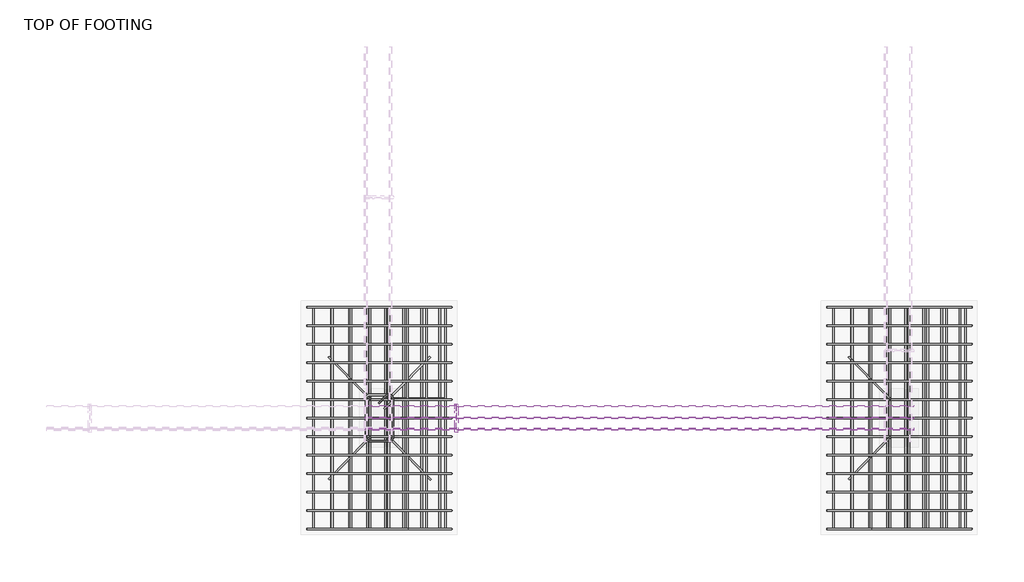
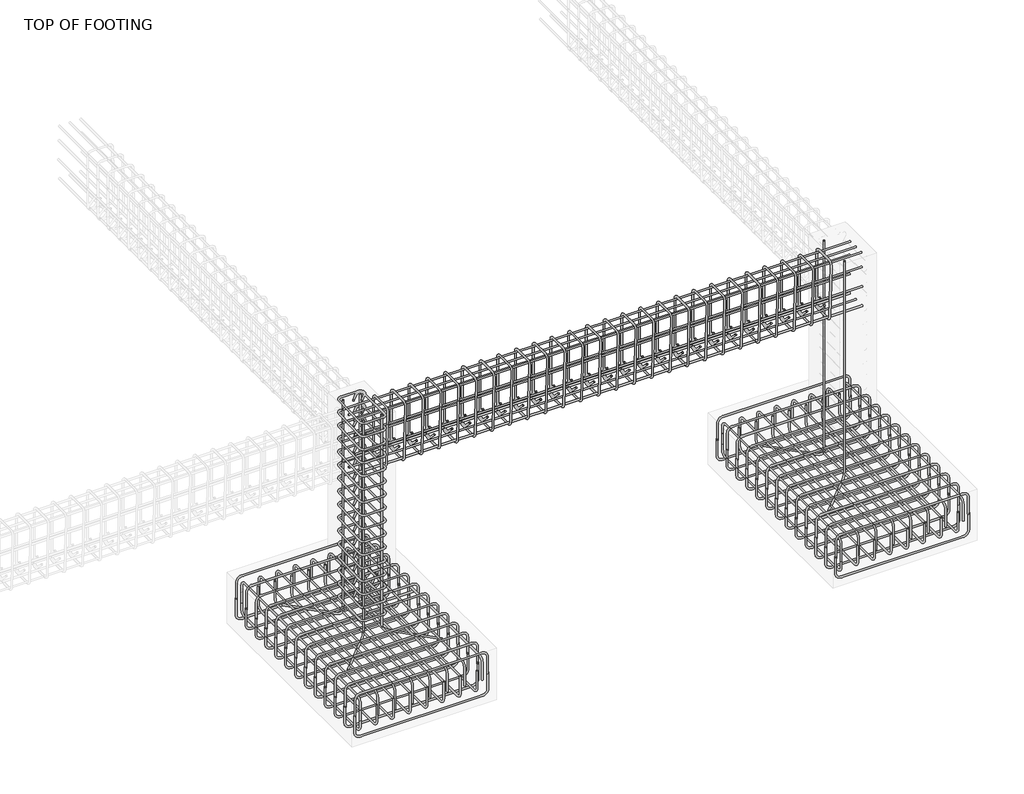
# One storey, part 4 of 21: 23 reinforcing bars.
"""IFC4 building model written with IfcOpenShell, lengths in millimetres."""

from ifc_helpers import new_model, si_unit, point, frame, origin, place, context, project, spatial, polyline, circle_curve, trimmed, segment, composite_curve, source, transform, mapped, element, save
from ifc_brep_helpers import swept_disk

model = new_model("IFC4")

# Units and contexts
model_context = context("Model", 3, world=origin())
ifc_project = project(units=[si_unit("LENGTHUNIT", "METRE", prefix="MILLI")], contexts=[model_context])

# Site, building, storey
site = spatial("IfcSite", under=ifc_project)
building = spatial("IfcBuilding", under=site)
storey = spatial("IfcBuildingStorey", under=building, Name="TOP OF FOOTING", Elevation=-1828.8)

# Reinforcing bars
placement = place(None, origin())
reinforcing_bar_shape = source(origin(), model_context, "Body", "SolidModel", [
    swept_disk(composite_curve([segment(polyline([(-1248.5313539, 443.1886958, -2045.4168622), (-1248.5313539, 443.1886958, -2192.7168622)]), True, "CONTINUOUS"), segment(trimmed(circle_curve(frame((-1294.8813539, 443.1886958, -2192.7168622), z_axis=(0.0, 1.0, 0.0), x_axis=(46.34999999999991, 0.0, 0.0)), 46.35), [point((-1248.5313539, 443.1886958, -2192.7168622))], [point((-1294.8813539, 443.1886958, -2239.0668622))], True, "CARTESIAN"), True, "CONTINUOUS"), segment(polyline([(-1294.8813539, 443.1886958, -2239.0668622), (-2309.4813539, 443.1886958, -2239.0668622)]), True, "CONTINUOUS"), segment(trimmed(circle_curve(frame((-2309.4813539, 443.1886958, -2192.7168622), z_axis=(0.0, 1.0, 0.0), x_axis=(0.0, 0.0, -46.34999999999991)), 46.35), [point((-2309.4813539, 443.1886958, -2239.0668622))], [point((-2355.8313539, 443.1886958, -2192.7168622))], True, "CARTESIAN"), True, "CONTINUOUS"), segment(polyline([(-2355.8313539, 443.1886958, -2192.7168622), (-2355.8313539, 443.1886958, -2045.4168622)]), True, "CONTINUOUS")], self_intersect=False), 6.35),
])
element("IfcReinforcingBar", 1, at=placement, inside=storey, context=model_context, shape_type="MappedRepresentation", body=[
    mapped(reinforcing_bar_shape, transform((0.0, 0.0, 0.0), x_axis=(1.0, 0.0, 0.0), y_axis=(0.0, 1.0, 0.0), z_axis=(0.0, 0.0, 1.0))),
    mapped(reinforcing_bar_shape, transform((0.0, -142.275, 0.0), x_axis=(1.0, 0.0, 0.0), y_axis=(0.0, 1.0, 0.0), z_axis=(0.0, 0.0, 1.0))),
    mapped(reinforcing_bar_shape, transform((0.0, -284.55, 0.0), x_axis=(1.0, 0.0, 0.0), y_axis=(0.0, 1.0, 0.0), z_axis=(0.0, 0.0, 1.0))),
    mapped(reinforcing_bar_shape, transform((0.0, -426.825, 0.0), x_axis=(1.0, 0.0, 0.0), y_axis=(0.0, 1.0, 0.0), z_axis=(0.0, 0.0, 1.0))),
    mapped(reinforcing_bar_shape, transform((0.0, -569.1, 0.0), x_axis=(1.0, 0.0, 0.0), y_axis=(0.0, 1.0, 0.0), z_axis=(0.0, 0.0, 1.0))),
    mapped(reinforcing_bar_shape, transform((0.0, -711.375, 0.0), x_axis=(1.0, 0.0, 0.0), y_axis=(0.0, 1.0, 0.0), z_axis=(0.0, 0.0, 1.0))),
    mapped(reinforcing_bar_shape, transform((0.0, -853.65, 0.0), x_axis=(1.0, 0.0, 0.0), y_axis=(0.0, 1.0, 0.0), z_axis=(0.0, 0.0, 1.0))),
    mapped(reinforcing_bar_shape, transform((0.0, -995.925, 0.0), x_axis=(1.0, 0.0, 0.0), y_axis=(0.0, 1.0, 0.0), z_axis=(0.0, 0.0, 1.0))),
    mapped(reinforcing_bar_shape, transform((0.0, -1138.2, 0.0), x_axis=(1.0, 0.0, 0.0), y_axis=(0.0, 1.0, 0.0), z_axis=(0.0, 0.0, 1.0))),
    mapped(reinforcing_bar_shape, transform((0.0, -1280.475, 0.0), x_axis=(1.0, 0.0, 0.0), y_axis=(0.0, 1.0, 0.0), z_axis=(0.0, 0.0, 1.0))),
    mapped(reinforcing_bar_shape, transform((0.0, -1422.75, 0.0), x_axis=(1.0, 0.0, 0.0), y_axis=(0.0, 1.0, 0.0), z_axis=(0.0, 0.0, 1.0))),
    mapped(reinforcing_bar_shape, transform((0.0, -1565.025, 0.0), x_axis=(1.0, 0.0, 0.0), y_axis=(0.0, 1.0, 0.0), z_axis=(0.0, 0.0, 1.0))),
    mapped(reinforcing_bar_shape, transform((0.0, -1707.3, 0.0), x_axis=(1.0, 0.0, 0.0), y_axis=(0.0, 1.0, 0.0), z_axis=(0.0, 0.0, 1.0))),
])
reinforcing_bar_2_shape = source(origin(), model_context, "Body", "SolidModel", [
    swept_disk(composite_curve([segment(polyline([(-2352.5002917, 443.1886958, -2057.1074344), (-2352.5002917, 443.1886958, -1909.8074344)]), True, "CONTINUOUS"), segment(trimmed(circle_curve(frame((-2306.1502917, 443.1886958, -1909.8074344), z_axis=(0.0, 1.0, 0.0), x_axis=(-46.350000000000364, 0.0, 0.0)), 46.35), [point((-2352.5002917, 443.1886958, -1909.8074344))], [point((-2306.1502917, 443.1886958, -1863.4574344))], True, "CARTESIAN"), True, "CONTINUOUS"), segment(polyline([(-2306.1502917, 443.1886958, -1863.4574344), (-1297.2599214, 443.1886958, -1863.4574344)]), True, "CONTINUOUS"), segment(trimmed(circle_curve(frame((-1297.2599214, 443.1886958, -1909.8074344), z_axis=(0.0, 1.0, 0.0), x_axis=(0.0, 0.0, 46.34999999999991)), 46.35), [point((-1297.2599214, 443.1886958, -1863.4574344))], [point((-1250.9099214, 443.1886958, -1909.8074344))], True, "CARTESIAN"), True, "CONTINUOUS"), segment(polyline([(-1250.9099214, 443.1886958, -1909.8074344), (-1250.9099214, 443.1886958, -2057.1074344)]), True, "CONTINUOUS")], self_intersect=False), 6.35),
])
element("IfcReinforcingBar", 2, at=placement, inside=storey, context=model_context, shape_type="MappedRepresentation", body=[
    mapped(reinforcing_bar_2_shape, transform((0.0, 0.0, 0.0), x_axis=(1.0, 0.0, 0.0), y_axis=(0.0, 1.0, 0.0), z_axis=(0.0, 0.0, 1.0))),
    mapped(reinforcing_bar_2_shape, transform((0.0, -142.275, 0.0), x_axis=(1.0, 0.0, 0.0), y_axis=(0.0, 1.0, 0.0), z_axis=(0.0, 0.0, 1.0))),
    mapped(reinforcing_bar_2_shape, transform((0.0, -284.55, 0.0), x_axis=(1.0, 0.0, 0.0), y_axis=(0.0, 1.0, 0.0), z_axis=(0.0, 0.0, 1.0))),
    mapped(reinforcing_bar_2_shape, transform((0.0, -426.825, 0.0), x_axis=(1.0, 0.0, 0.0), y_axis=(0.0, 1.0, 0.0), z_axis=(0.0, 0.0, 1.0))),
    mapped(reinforcing_bar_2_shape, transform((0.0, -569.1, 0.0), x_axis=(1.0, 0.0, 0.0), y_axis=(0.0, 1.0, 0.0), z_axis=(0.0, 0.0, 1.0))),
    mapped(reinforcing_bar_2_shape, transform((0.0, -711.375, 0.0), x_axis=(1.0, 0.0, 0.0), y_axis=(0.0, 1.0, 0.0), z_axis=(0.0, 0.0, 1.0))),
    mapped(reinforcing_bar_2_shape, transform((0.0, -853.65, 0.0), x_axis=(1.0, 0.0, 0.0), y_axis=(0.0, 1.0, 0.0), z_axis=(0.0, 0.0, 1.0))),
    mapped(reinforcing_bar_2_shape, transform((0.0, -995.925, 0.0), x_axis=(1.0, 0.0, 0.0), y_axis=(0.0, 1.0, 0.0), z_axis=(0.0, 0.0, 1.0))),
    mapped(reinforcing_bar_2_shape, transform((0.0, -1138.2, 0.0), x_axis=(1.0, 0.0, 0.0), y_axis=(0.0, 1.0, 0.0), z_axis=(0.0, 0.0, 1.0))),
    mapped(reinforcing_bar_2_shape, transform((0.0, -1280.475, 0.0), x_axis=(1.0, 0.0, 0.0), y_axis=(0.0, 1.0, 0.0), z_axis=(0.0, 0.0, 1.0))),
    mapped(reinforcing_bar_2_shape, transform((0.0, -1422.75, 0.0), x_axis=(1.0, 0.0, 0.0), y_axis=(0.0, 1.0, 0.0), z_axis=(0.0, 0.0, 1.0))),
    mapped(reinforcing_bar_2_shape, transform((0.0, -1565.025, 0.0), x_axis=(1.0, 0.0, 0.0), y_axis=(0.0, 1.0, 0.0), z_axis=(0.0, 0.0, 1.0))),
    mapped(reinforcing_bar_2_shape, transform((0.0, -1707.3, 0.0), x_axis=(1.0, 0.0, 0.0), y_axis=(0.0, 1.0, 0.0), z_axis=(0.0, 0.0, 1.0))),
])
reinforcing_bar_3_shape = source(origin(), model_context, "Body", "SolidModel", [
    swept_disk(composite_curve([segment(polyline([(-1294.4849216, 443.1886958, -2099.3509187), (-1294.4849216, 443.1886958, -1952.0509187)]), True, "CONTINUOUS"), segment(trimmed(circle_curve(frame((-1294.4849216, 396.8386958, -1952.0509187), z_axis=(1.0, 0.0, 0.0), x_axis=(0.0, 46.35000000000002, 0.0)), 46.35), [point((-1294.4849216, 443.1886958, -1952.0509187))], [point((-1294.4849216, 396.8386958, -1905.7009187))], True, "CARTESIAN"), True, "CONTINUOUS"), segment(polyline([(-1294.4849216, 396.8386958, -1905.7009187), (-1294.4849216, -1217.7613042, -1905.7009187)]), True, "CONTINUOUS"), segment(trimmed(circle_curve(frame((-1294.4849216, -1217.7613042, -1952.0509187), z_axis=(1.0, 0.0, 0.0), x_axis=(0.0, 0.0, 46.34999999999991)), 46.35), [point((-1294.4849216, -1217.7613042, -1905.7009187))], [point((-1294.4849216, -1264.1113042, -1952.0509187))], True, "CARTESIAN"), True, "CONTINUOUS"), segment(polyline([(-1294.4849216, -1264.1113042, -1952.0509187), (-1294.4849216, -1264.1113042, -2099.3509187)]), True, "CONTINUOUS")], self_intersect=False), 6.35),
])
element("IfcReinforcingBar", 3, at=placement, inside=storey, context=model_context, shape_type="MappedRepresentation", body=[
    mapped(reinforcing_bar_3_shape, transform((0.0, 0.0, 0.0), x_axis=(1.0, 0.0, 0.0), y_axis=(0.0, 1.0, 0.0), z_axis=(0.0, 0.0, 1.0))),
    mapped(reinforcing_bar_3_shape, transform((-145.0295561, 0.0, 0.0), x_axis=(1.0, 0.0, 0.0), y_axis=(0.0, 1.0, 0.0), z_axis=(0.0, 0.0, 1.0))),
    mapped(reinforcing_bar_3_shape, transform((-290.0591123, 0.0, 0.0), x_axis=(1.0, 0.0, 0.0), y_axis=(0.0, 1.0, 0.0), z_axis=(0.0, 0.0, 1.0))),
    mapped(reinforcing_bar_3_shape, transform((-435.0886684, 0.0, 0.0), x_axis=(1.0, 0.0, 0.0), y_axis=(0.0, 1.0, 0.0), z_axis=(0.0, 0.0, 1.0))),
    mapped(reinforcing_bar_3_shape, transform((-580.1182245, 0.0, 0.0), x_axis=(1.0, 0.0, 0.0), y_axis=(0.0, 1.0, 0.0), z_axis=(0.0, 0.0, 1.0))),
    mapped(reinforcing_bar_3_shape, transform((-725.1477807, 0.0, 0.0), x_axis=(1.0, 0.0, 0.0), y_axis=(0.0, 1.0, 0.0), z_axis=(0.0, 0.0, 1.0))),
    mapped(reinforcing_bar_3_shape, transform((-870.1773368, 0.0, 0.0), x_axis=(1.0, 0.0, 0.0), y_axis=(0.0, 1.0, 0.0), z_axis=(0.0, 0.0, 1.0))),
    mapped(reinforcing_bar_3_shape, transform((-1015.206893, 0.0, 0.0), x_axis=(1.0, 0.0, 0.0), y_axis=(0.0, 1.0, 0.0), z_axis=(0.0, 0.0, 1.0))),
])
reinforcing_bar_4_shape = source(origin(), model_context, "Body", "SolidModel", [
    swept_disk(composite_curve([segment(polyline([(-2309.6918146, 443.1886958, -2006.0306816), (-2309.6918146, 443.1886958, -2153.3306816)]), True, "CONTINUOUS"), segment(trimmed(circle_curve(frame((-2309.6918146, 396.8386958, -2153.3306816), z_axis=(-1.0, 0.0, 0.0), x_axis=(0.0, 46.35000000000002, 0.0)), 46.35), [point((-2309.6918146, 443.1886958, -2153.3306816))], [point((-2309.6918146, 396.8386958, -2199.6806816))], True, "CARTESIAN"), True, "CONTINUOUS"), segment(polyline([(-2309.6918146, 396.8386958, -2199.6806816), (-2309.6918146, -1217.7613042, -2199.6806816)]), True, "CONTINUOUS"), segment(trimmed(circle_curve(frame((-2309.6918146, -1217.7613042, -2153.3306816), z_axis=(-1.0, 0.0, 0.0), x_axis=(0.0, 0.0, -46.34999999999991)), 46.35), [point((-2309.6918146, -1217.7613042, -2199.6806816))], [point((-2309.6918146, -1264.1113042, -2153.3306816))], True, "CARTESIAN"), True, "CONTINUOUS"), segment(polyline([(-2309.6918146, -1264.1113042, -2153.3306816), (-2309.6918146, -1264.1113042, -2006.0306816)]), True, "CONTINUOUS")], self_intersect=False), 6.35),
])
element("IfcReinforcingBar", 4, at=placement, inside=storey, context=model_context, shape_type="MappedRepresentation", body=[
    mapped(reinforcing_bar_4_shape, transform((0.0, 0.0, 0.0), x_axis=(1.0, 0.0, 0.0), y_axis=(0.0, 1.0, 0.0), z_axis=(0.0, 0.0, 1.0))),
    mapped(reinforcing_bar_4_shape, transform((138.8823255, 0.0, 0.0), x_axis=(1.0, 0.0, 0.0), y_axis=(0.0, 1.0, 0.0), z_axis=(0.0, 0.0, 1.0))),
    mapped(reinforcing_bar_4_shape, transform((277.7646509, 0.0, 0.0), x_axis=(1.0, 0.0, 0.0), y_axis=(0.0, 1.0, 0.0), z_axis=(0.0, 0.0, 1.0))),
    mapped(reinforcing_bar_4_shape, transform((416.6469764, 0.0, 0.0), x_axis=(1.0, 0.0, 0.0), y_axis=(0.0, 1.0, 0.0), z_axis=(0.0, 0.0, 1.0))),
    mapped(reinforcing_bar_4_shape, transform((555.5293018, 0.0, 0.0), x_axis=(1.0, 0.0, 0.0), y_axis=(0.0, 1.0, 0.0), z_axis=(0.0, 0.0, 1.0))),
    mapped(reinforcing_bar_4_shape, transform((694.4116273, 0.0, 0.0), x_axis=(1.0, 0.0, 0.0), y_axis=(0.0, 1.0, 0.0), z_axis=(0.0, 0.0, 1.0))),
    mapped(reinforcing_bar_4_shape, transform((833.2939527, 0.0, 0.0), x_axis=(1.0, 0.0, 0.0), y_axis=(0.0, 1.0, 0.0), z_axis=(0.0, 0.0, 1.0))),
    mapped(reinforcing_bar_4_shape, transform((972.1762782, 0.0, 0.0), x_axis=(1.0, 0.0, 0.0), y_axis=(0.0, 1.0, 0.0), z_axis=(0.0, 0.0, 1.0))),
])
reinforcing_bar_5_shape = source(origin(), model_context, "Body", "SolidModel", [
    swept_disk(composite_curve([segment(polyline([(2751.4686461, 443.1886958, -2045.4168622), (2751.4686461, 443.1886958, -2192.7168622)]), True, "CONTINUOUS"), segment(trimmed(circle_curve(frame((2705.1186461, 443.1886958, -2192.7168622), z_axis=(0.0, 1.0, 0.0), x_axis=(46.34999999999991, 0.0, 0.0)), 46.35), [point((2751.4686461, 443.1886958, -2192.7168622))], [point((2705.1186461, 443.1886958, -2239.0668622))], True, "CARTESIAN"), True, "CONTINUOUS"), segment(polyline([(2705.1186461, 443.1886958, -2239.0668622), (1690.5186461, 443.1886958, -2239.0668622)]), True, "CONTINUOUS"), segment(trimmed(circle_curve(frame((1690.5186461, 443.1886958, -2192.7168622), z_axis=(0.0, 1.0, 0.0), x_axis=(0.0, 0.0, -46.34999999999991)), 46.35), [point((1690.5186461, 443.1886958, -2239.0668622))], [point((1644.1686461, 443.1886958, -2192.7168622))], True, "CARTESIAN"), True, "CONTINUOUS"), segment(polyline([(1644.1686461, 443.1886958, -2192.7168622), (1644.1686461, 443.1886958, -2045.4168622)]), True, "CONTINUOUS")], self_intersect=False), 6.35),
])
element("IfcReinforcingBar", 5, at=placement, inside=storey, context=model_context, shape_type="MappedRepresentation", body=[
    mapped(reinforcing_bar_5_shape, transform((0.0, 0.0, 0.0), x_axis=(1.0, 0.0, 0.0), y_axis=(0.0, 1.0, 0.0), z_axis=(0.0, 0.0, 1.0))),
    mapped(reinforcing_bar_5_shape, transform((0.0, -142.275, 0.0), x_axis=(1.0, 0.0, 0.0), y_axis=(0.0, 1.0, 0.0), z_axis=(0.0, 0.0, 1.0))),
    mapped(reinforcing_bar_5_shape, transform((0.0, -284.55, 0.0), x_axis=(1.0, 0.0, 0.0), y_axis=(0.0, 1.0, 0.0), z_axis=(0.0, 0.0, 1.0))),
    mapped(reinforcing_bar_5_shape, transform((0.0, -426.825, 0.0), x_axis=(1.0, 0.0, 0.0), y_axis=(0.0, 1.0, 0.0), z_axis=(0.0, 0.0, 1.0))),
    mapped(reinforcing_bar_5_shape, transform((0.0, -569.1, 0.0), x_axis=(1.0, 0.0, 0.0), y_axis=(0.0, 1.0, 0.0), z_axis=(0.0, 0.0, 1.0))),
    mapped(reinforcing_bar_5_shape, transform((0.0, -711.375, 0.0), x_axis=(1.0, 0.0, 0.0), y_axis=(0.0, 1.0, 0.0), z_axis=(0.0, 0.0, 1.0))),
    mapped(reinforcing_bar_5_shape, transform((0.0, -853.65, 0.0), x_axis=(1.0, 0.0, 0.0), y_axis=(0.0, 1.0, 0.0), z_axis=(0.0, 0.0, 1.0))),
    mapped(reinforcing_bar_5_shape, transform((0.0, -995.925, 0.0), x_axis=(1.0, 0.0, 0.0), y_axis=(0.0, 1.0, 0.0), z_axis=(0.0, 0.0, 1.0))),
    mapped(reinforcing_bar_5_shape, transform((0.0, -1138.2, 0.0), x_axis=(1.0, 0.0, 0.0), y_axis=(0.0, 1.0, 0.0), z_axis=(0.0, 0.0, 1.0))),
    mapped(reinforcing_bar_5_shape, transform((0.0, -1280.475, 0.0), x_axis=(1.0, 0.0, 0.0), y_axis=(0.0, 1.0, 0.0), z_axis=(0.0, 0.0, 1.0))),
    mapped(reinforcing_bar_5_shape, transform((0.0, -1422.75, 0.0), x_axis=(1.0, 0.0, 0.0), y_axis=(0.0, 1.0, 0.0), z_axis=(0.0, 0.0, 1.0))),
    mapped(reinforcing_bar_5_shape, transform((0.0, -1565.025, 0.0), x_axis=(1.0, 0.0, 0.0), y_axis=(0.0, 1.0, 0.0), z_axis=(0.0, 0.0, 1.0))),
    mapped(reinforcing_bar_5_shape, transform((0.0, -1707.3, 0.0), x_axis=(1.0, 0.0, 0.0), y_axis=(0.0, 1.0, 0.0), z_axis=(0.0, 0.0, 1.0))),
])
reinforcing_bar_6_shape = source(origin(), model_context, "Body", "SolidModel", [
    swept_disk(composite_curve([segment(polyline([(1647.4997083, 443.1886958, -2057.1074344), (1647.4997083, 443.1886958, -1909.8074344)]), True, "CONTINUOUS"), segment(trimmed(circle_curve(frame((1693.8497083, 443.1886958, -1909.8074344), z_axis=(0.0, 1.0, 0.0), x_axis=(-46.34999999999991, 0.0, 0.0)), 46.35), [point((1647.4997083, 443.1886958, -1909.8074344))], [point((1693.8497083, 443.1886958, -1863.4574344))], True, "CARTESIAN"), True, "CONTINUOUS"), segment(polyline([(1693.8497083, 443.1886958, -1863.4574344), (2702.7400786, 443.1886958, -1863.4574344)]), True, "CONTINUOUS"), segment(trimmed(circle_curve(frame((2702.7400786, 443.1886958, -1909.8074344), z_axis=(0.0, 1.0, 0.0), x_axis=(0.0, 0.0, 46.34999999999991)), 46.35), [point((2702.7400786, 443.1886958, -1863.4574344))], [point((2749.0900786, 443.1886958, -1909.8074344))], True, "CARTESIAN"), True, "CONTINUOUS"), segment(polyline([(2749.0900786, 443.1886958, -1909.8074344), (2749.0900786, 443.1886958, -2057.1074344)]), True, "CONTINUOUS")], self_intersect=False), 6.35),
])
element("IfcReinforcingBar", 6, at=placement, inside=storey, context=model_context, shape_type="MappedRepresentation", body=[
    mapped(reinforcing_bar_6_shape, transform((0.0, 0.0, 0.0), x_axis=(1.0, 0.0, 0.0), y_axis=(0.0, 1.0, 0.0), z_axis=(0.0, 0.0, 1.0))),
    mapped(reinforcing_bar_6_shape, transform((0.0, -142.275, 0.0), x_axis=(1.0, 0.0, 0.0), y_axis=(0.0, 1.0, 0.0), z_axis=(0.0, 0.0, 1.0))),
    mapped(reinforcing_bar_6_shape, transform((0.0, -284.55, 0.0), x_axis=(1.0, 0.0, 0.0), y_axis=(0.0, 1.0, 0.0), z_axis=(0.0, 0.0, 1.0))),
    mapped(reinforcing_bar_6_shape, transform((0.0, -426.825, 0.0), x_axis=(1.0, 0.0, 0.0), y_axis=(0.0, 1.0, 0.0), z_axis=(0.0, 0.0, 1.0))),
    mapped(reinforcing_bar_6_shape, transform((0.0, -569.1, 0.0), x_axis=(1.0, 0.0, 0.0), y_axis=(0.0, 1.0, 0.0), z_axis=(0.0, 0.0, 1.0))),
    mapped(reinforcing_bar_6_shape, transform((0.0, -711.375, 0.0), x_axis=(1.0, 0.0, 0.0), y_axis=(0.0, 1.0, 0.0), z_axis=(0.0, 0.0, 1.0))),
    mapped(reinforcing_bar_6_shape, transform((0.0, -853.65, 0.0), x_axis=(1.0, 0.0, 0.0), y_axis=(0.0, 1.0, 0.0), z_axis=(0.0, 0.0, 1.0))),
    mapped(reinforcing_bar_6_shape, transform((0.0, -995.925, 0.0), x_axis=(1.0, 0.0, 0.0), y_axis=(0.0, 1.0, 0.0), z_axis=(0.0, 0.0, 1.0))),
    mapped(reinforcing_bar_6_shape, transform((0.0, -1138.2, 0.0), x_axis=(1.0, 0.0, 0.0), y_axis=(0.0, 1.0, 0.0), z_axis=(0.0, 0.0, 1.0))),
    mapped(reinforcing_bar_6_shape, transform((0.0, -1280.475, 0.0), x_axis=(1.0, 0.0, 0.0), y_axis=(0.0, 1.0, 0.0), z_axis=(0.0, 0.0, 1.0))),
    mapped(reinforcing_bar_6_shape, transform((0.0, -1422.75, 0.0), x_axis=(1.0, 0.0, 0.0), y_axis=(0.0, 1.0, 0.0), z_axis=(0.0, 0.0, 1.0))),
    mapped(reinforcing_bar_6_shape, transform((0.0, -1565.025, 0.0), x_axis=(1.0, 0.0, 0.0), y_axis=(0.0, 1.0, 0.0), z_axis=(0.0, 0.0, 1.0))),
    mapped(reinforcing_bar_6_shape, transform((0.0, -1707.3, 0.0), x_axis=(1.0, 0.0, 0.0), y_axis=(0.0, 1.0, 0.0), z_axis=(0.0, 0.0, 1.0))),
])
reinforcing_bar_7_shape = source(origin(), model_context, "Body", "SolidModel", [
    swept_disk(composite_curve([segment(polyline([(2705.5150784, 443.1886958, -2099.3509187), (2705.5150784, 443.1886958, -1952.0509187)]), True, "CONTINUOUS"), segment(trimmed(circle_curve(frame((2705.5150784, 396.8386958, -1952.0509187), z_axis=(1.0, 0.0, 0.0), x_axis=(0.0, 46.35000000000002, 0.0)), 46.35), [point((2705.5150784, 443.1886958, -1952.0509187))], [point((2705.5150784, 396.8386958, -1905.7009187))], True, "CARTESIAN"), True, "CONTINUOUS"), segment(polyline([(2705.5150784, 396.8386958, -1905.7009187), (2705.5150784, -1217.7613042, -1905.7009187)]), True, "CONTINUOUS"), segment(trimmed(circle_curve(frame((2705.5150784, -1217.7613042, -1952.0509187), z_axis=(1.0, 0.0, 0.0), x_axis=(0.0, 0.0, 46.34999999999991)), 46.35), [point((2705.5150784, -1217.7613042, -1905.7009187))], [point((2705.5150784, -1264.1113042, -1952.0509187))], True, "CARTESIAN"), True, "CONTINUOUS"), segment(polyline([(2705.5150784, -1264.1113042, -1952.0509187), (2705.5150784, -1264.1113042, -2099.3509187)]), True, "CONTINUOUS")], self_intersect=False), 6.35),
])
element("IfcReinforcingBar", 7, at=placement, inside=storey, context=model_context, shape_type="MappedRepresentation", body=[
    mapped(reinforcing_bar_7_shape, transform((0.0, 0.0, 0.0), x_axis=(1.0, 0.0, 0.0), y_axis=(0.0, 1.0, 0.0), z_axis=(0.0, 0.0, 1.0))),
    mapped(reinforcing_bar_7_shape, transform((-145.0295561, 0.0, 0.0), x_axis=(1.0, 0.0, 0.0), y_axis=(0.0, 1.0, 0.0), z_axis=(0.0, 0.0, 1.0))),
    mapped(reinforcing_bar_7_shape, transform((-290.0591123, 0.0, 0.0), x_axis=(1.0, 0.0, 0.0), y_axis=(0.0, 1.0, 0.0), z_axis=(0.0, 0.0, 1.0))),
    mapped(reinforcing_bar_7_shape, transform((-435.0886684, 0.0, 0.0), x_axis=(1.0, 0.0, 0.0), y_axis=(0.0, 1.0, 0.0), z_axis=(0.0, 0.0, 1.0))),
    mapped(reinforcing_bar_7_shape, transform((-580.1182245, 0.0, 0.0), x_axis=(1.0, 0.0, 0.0), y_axis=(0.0, 1.0, 0.0), z_axis=(0.0, 0.0, 1.0))),
    mapped(reinforcing_bar_7_shape, transform((-725.1477807, 0.0, 0.0), x_axis=(1.0, 0.0, 0.0), y_axis=(0.0, 1.0, 0.0), z_axis=(0.0, 0.0, 1.0))),
    mapped(reinforcing_bar_7_shape, transform((-870.1773368, 0.0, 0.0), x_axis=(1.0, 0.0, 0.0), y_axis=(0.0, 1.0, 0.0), z_axis=(0.0, 0.0, 1.0))),
    mapped(reinforcing_bar_7_shape, transform((-1015.206893, 0.0, 0.0), x_axis=(1.0, 0.0, 0.0), y_axis=(0.0, 1.0, 0.0), z_axis=(0.0, 0.0, 1.0))),
])
reinforcing_bar_8_shape = source(origin(), model_context, "Body", "SolidModel", [
    swept_disk(composite_curve([segment(polyline([(1690.3081854, 443.1886958, -2006.0306816), (1690.3081854, 443.1886958, -2153.3306816)]), True, "CONTINUOUS"), segment(trimmed(circle_curve(frame((1690.3081854, 396.8386958, -2153.3306816), z_axis=(-1.0, 0.0, 0.0), x_axis=(0.0, 46.35000000000002, 0.0)), 46.35), [point((1690.3081854, 443.1886958, -2153.3306816))], [point((1690.3081854, 396.8386958, -2199.6806816))], True, "CARTESIAN"), True, "CONTINUOUS"), segment(polyline([(1690.3081854, 396.8386958, -2199.6806816), (1690.3081854, -1217.7613042, -2199.6806816)]), True, "CONTINUOUS"), segment(trimmed(circle_curve(frame((1690.3081854, -1217.7613042, -2153.3306816), z_axis=(-1.0, 0.0, 0.0), x_axis=(0.0, 0.0, -46.34999999999991)), 46.35), [point((1690.3081854, -1217.7613042, -2199.6806816))], [point((1690.3081854, -1264.1113042, -2153.3306816))], True, "CARTESIAN"), True, "CONTINUOUS"), segment(polyline([(1690.3081854, -1264.1113042, -2153.3306816), (1690.3081854, -1264.1113042, -2006.0306816)]), True, "CONTINUOUS")], self_intersect=False), 6.35),
])
element("IfcReinforcingBar", 8, at=placement, inside=storey, context=model_context, shape_type="MappedRepresentation", body=[
    mapped(reinforcing_bar_8_shape, transform((0.0, 0.0, 0.0), x_axis=(1.0, 0.0, 0.0), y_axis=(0.0, 1.0, 0.0), z_axis=(0.0, 0.0, 1.0))),
    mapped(reinforcing_bar_8_shape, transform((138.8823255, 0.0, 0.0), x_axis=(1.0, 0.0, 0.0), y_axis=(0.0, 1.0, 0.0), z_axis=(0.0, 0.0, 1.0))),
    mapped(reinforcing_bar_8_shape, transform((277.7646509, 0.0, 0.0), x_axis=(1.0, 0.0, 0.0), y_axis=(0.0, 1.0, 0.0), z_axis=(0.0, 0.0, 1.0))),
    mapped(reinforcing_bar_8_shape, transform((416.6469764, 0.0, 0.0), x_axis=(1.0, 0.0, 0.0), y_axis=(0.0, 1.0, 0.0), z_axis=(0.0, 0.0, 1.0))),
    mapped(reinforcing_bar_8_shape, transform((555.5293018, 0.0, 0.0), x_axis=(1.0, 0.0, 0.0), y_axis=(0.0, 1.0, 0.0), z_axis=(0.0, 0.0, 1.0))),
    mapped(reinforcing_bar_8_shape, transform((694.4116273, 0.0, 0.0), x_axis=(1.0, 0.0, 0.0), y_axis=(0.0, 1.0, 0.0), z_axis=(0.0, 0.0, 1.0))),
    mapped(reinforcing_bar_8_shape, transform((833.2939527, 0.0, 0.0), x_axis=(1.0, 0.0, 0.0), y_axis=(0.0, 1.0, 0.0), z_axis=(0.0, 0.0, 1.0))),
    mapped(reinforcing_bar_8_shape, transform((972.1762782, 0.0, 0.0), x_axis=(1.0, 0.0, 0.0), y_axis=(0.0, 1.0, 0.0), z_axis=(0.0, 0.0, 1.0))),
])
reinforcing_bar_9_shape = source(origin(), model_context, "Body", "SolidModel", [
    swept_disk(composite_curve([segment(polyline([(-1807.7927145, -296.7370695, -46.35), (-1752.0491515, -240.9935066, -46.35)]), True, "CONTINUOUS"), segment(trimmed(circle_curve(frame((-1729.8813539, -263.1613042, -46.35), z_axis=(0.0, 0.0, -1.0), x_axis=(-22.167797600000085, 22.16779760000003, 0.0)), 31.35), [point((-1752.0491515, -240.9935066, -46.35))], [point((-1698.5313539, -263.1613042, -46.35))], True, "CARTESIAN"), True, "CONTINUOUS"), segment(polyline([(-1698.5313539, -263.1613042, -46.35), (-1698.5313539, -557.7613042, -46.35)]), True, "CONTINUOUS"), segment(trimmed(circle_curve(frame((-1729.8813539, -557.7613042, -46.35), z_axis=(0.0, 0.0, -1.0), x_axis=(31.34999999999991, 0.0, 0.0)), 31.35), [point((-1698.5313539, -557.7613042, -46.35))], [point((-1729.8813539, -589.1113042, -46.35))], True, "CARTESIAN"), True, "CONTINUOUS"), segment(polyline([(-1729.8813539, -589.1113042, -46.35), (-1874.4813539, -589.1113042, -46.35)]), True, "CONTINUOUS"), segment(trimmed(circle_curve(frame((-1874.4813539, -557.7810893, -45.2363875), z_axis=(0.0, 0.035521928334481916, -0.9993688971583016), x_axis=(0.0, -31.330214899999987, -1.1136125000000021)), 31.35), [point((-1874.4813539, -589.1113042, -46.35))], [point((-1905.8313539, -557.7810893, -45.2363875))], True, "CARTESIAN"), True, "CONTINUOUS"), segment(polyline([(-1905.8313539, -557.7810893, -45.2363875), (-1905.8313539, -263.1415191, -34.7636125)]), True, "CONTINUOUS"), segment(trimmed(circle_curve(frame((-1874.4813539, -263.1415191, -34.7636125), z_axis=(0.0, 0.035521928334481916, -0.9993688971583016), x_axis=(-31.350000000000136, 0.0, 0.0)), 31.35), [point((-1905.8313539, -263.1415191, -34.7636125))], [point((-1874.4813539, -231.8113042, -33.65))], True, "CARTESIAN"), True, "CONTINUOUS"), segment(polyline([(-1874.4813539, -231.8113042, -33.65), (-1729.8813539, -231.8113042, -33.65)]), True, "CONTINUOUS"), segment(trimmed(circle_curve(frame((-1729.8813539, -263.1613042, -33.65), z_axis=(0.0, 0.0, -1.0), x_axis=(0.0, 31.350000000000023, 0.0)), 31.35), [point((-1729.8813539, -231.8113042, -33.65))], [point((-1707.7135563, -285.3291018, -33.65))], True, "CARTESIAN"), True, "CONTINUOUS"), segment(polyline([(-1707.7135563, -285.3291018, -33.65), (-1763.4571193, -341.0726647, -33.65)]), True, "CONTINUOUS")], self_intersect=False), 6.35),
])
element("IfcReinforcingBar", 9, at=placement, inside=storey, context=model_context, shape_type="MappedRepresentation", body=[
    mapped(reinforcing_bar_9_shape, transform((0.0, 0.0, 0.0), x_axis=(1.0, 0.0, 0.0), y_axis=(0.0, 1.0, 0.0), z_axis=(0.0, 0.0, 1.0))),
    mapped(reinforcing_bar_9_shape, transform((0.0, 0.0, -115.74), x_axis=(1.0, 0.0, 0.0), y_axis=(0.0, 1.0, 0.0), z_axis=(0.0, 0.0, 1.0))),
    mapped(reinforcing_bar_9_shape, transform((0.0, 0.0, -231.48), x_axis=(1.0, 0.0, 0.0), y_axis=(0.0, 1.0, 0.0), z_axis=(0.0, 0.0, 1.0))),
    mapped(reinforcing_bar_9_shape, transform((0.0, 0.0, -347.22), x_axis=(1.0, 0.0, 0.0), y_axis=(0.0, 1.0, 0.0), z_axis=(0.0, 0.0, 1.0))),
    mapped(reinforcing_bar_9_shape, transform((0.0, 0.0, -462.96), x_axis=(1.0, 0.0, 0.0), y_axis=(0.0, 1.0, 0.0), z_axis=(0.0, 0.0, 1.0))),
    mapped(reinforcing_bar_9_shape, transform((0.0, 0.0, -578.7), x_axis=(1.0, 0.0, 0.0), y_axis=(0.0, 1.0, 0.0), z_axis=(0.0, 0.0, 1.0))),
    mapped(reinforcing_bar_9_shape, transform((0.0, 0.0, -694.44), x_axis=(1.0, 0.0, 0.0), y_axis=(0.0, 1.0, 0.0), z_axis=(0.0, 0.0, 1.0))),
    mapped(reinforcing_bar_9_shape, transform((0.0, 0.0, -810.18), x_axis=(1.0, 0.0, 0.0), y_axis=(0.0, 1.0, 0.0), z_axis=(0.0, 0.0, 1.0))),
    mapped(reinforcing_bar_9_shape, transform((0.0, 0.0, -925.92), x_axis=(1.0, 0.0, 0.0), y_axis=(0.0, 1.0, 0.0), z_axis=(0.0, 0.0, 1.0))),
    mapped(reinforcing_bar_9_shape, transform((0.0, 0.0, -1041.66), x_axis=(1.0, 0.0, 0.0), y_axis=(0.0, 1.0, 0.0), z_axis=(0.0, 0.0, 1.0))),
    mapped(reinforcing_bar_9_shape, transform((0.0, 0.0, -1157.4), x_axis=(1.0, 0.0, 0.0), y_axis=(0.0, 1.0, 0.0), z_axis=(0.0, 0.0, 1.0))),
    mapped(reinforcing_bar_9_shape, transform((0.0, 0.0, -1273.14), x_axis=(1.0, 0.0, 0.0), y_axis=(0.0, 1.0, 0.0), z_axis=(0.0, 0.0, 1.0))),
    mapped(reinforcing_bar_9_shape, transform((0.0, 0.0, -1388.88), x_axis=(1.0, 0.0, 0.0), y_axis=(0.0, 1.0, 0.0), z_axis=(0.0, 0.0, 1.0))),
    mapped(reinforcing_bar_9_shape, transform((0.0, 0.0, -1504.62), x_axis=(1.0, 0.0, 0.0), y_axis=(0.0, 1.0, 0.0), z_axis=(0.0, 0.0, 1.0))),
    mapped(reinforcing_bar_9_shape, transform((0.0, 0.0, -1620.36), x_axis=(1.0, 0.0, 0.0), y_axis=(0.0, 1.0, 0.0), z_axis=(0.0, 0.0, 1.0))),
    mapped(reinforcing_bar_9_shape, transform((0.0, 0.0, -1736.1), x_axis=(1.0, 0.0, 0.0), y_axis=(0.0, 1.0, 0.0), z_axis=(0.0, 0.0, 1.0))),
])
element("IfcReinforcingBar", 10, at=placement, inside=storey, context=model_context, shape_type="SolidModel", body=[
    swept_disk(composite_curve([segment(polyline([(-1730.3607537, -262.059512, -40.0), (-1730.3607537, -262.059512, -1882.5259187)]), True, "CONTINUOUS"), segment(trimmed(circle_curve(frame((-1684.0107537, -262.059512, -1882.5259187), z_axis=(0.0, -1.0, 0.0), x_axis=(-46.350000000000136, 0.0, 0.0)), 46.35), [point((-1730.3607537, -262.059512, -1882.5259187))], [point((-1684.0107537, -262.059512, -1928.8759187))], True, "CARTESIAN"), True, "CONTINUOUS"), segment(polyline([(-1684.0107537, -262.059512, -1928.8759187), (-1294.4849216, -262.059512, -1928.8759187)]), True, "CONTINUOUS")], self_intersect=False), 6.35),
])
element("IfcReinforcingBar", 11, at=placement, inside=storey, context=model_context, shape_type="SolidModel", body=[
    swept_disk(composite_curve([segment(polyline([(-1730.3607537, -262.059512, -40.0), (-1730.3607537, -262.059512, -1882.5259187)]), True, "CONTINUOUS"), segment(trimmed(circle_curve(frame((-1697.9026361, -228.9718542, -1882.5259187), z_axis=(0.7138653253877265, -0.7002830122236834, 0.0), x_axis=(-32.45811759999992, -33.08765779999999, 0.0)), 46.35), [point((-1730.3607537, -262.059512, -1882.5259187))], [point((-1697.9026361, -228.9718542, -1928.8759187))], True, "CARTESIAN"), True, "CONTINUOUS"), segment(polyline([(-1697.9026361, -228.9718542, -1928.8759187), (-1413.1331156, 61.320903, -1928.8759187)]), True, "CONTINUOUS")], self_intersect=False), 6.35),
])
element("IfcReinforcingBar", 12, at=placement, inside=storey, context=model_context, shape_type="SolidModel", body=[
    swept_disk(composite_curve([segment(polyline([(-1874.0019542, -262.059512, -40.0), (-1874.0019542, -262.059512, -1882.5259187)]), True, "CONTINUOUS"), segment(trimmed(circle_curve(frame((-1906.4600718, -228.9718542, -1882.5259187), z_axis=(0.7138653253877092, 0.700283012223701, 0.0), x_axis=(32.45811759999992, -33.08765779999999, 0.0)), 46.35), [point((-1874.0019542, -262.059512, -1882.5259187))], [point((-1906.4600718, -228.9718542, -1928.8759187))], True, "CARTESIAN"), True, "CONTINUOUS"), segment(polyline([(-1906.4600718, -228.9718542, -1928.8759187), (-2191.2295922, 61.320903, -1928.8759187)]), True, "CONTINUOUS")], self_intersect=False), 6.35),
])
element("IfcReinforcingBar", 13, at=placement, inside=storey, context=model_context, shape_type="SolidModel", body=[
    swept_disk(composite_curve([segment(polyline([(-1725.3607537, -561.3630964, -40.0), (-1725.3607537, -561.3630964, -1882.5259187)]), True, "CONTINUOUS"), segment(trimmed(circle_curve(frame((-1692.9026361, -594.4507542, -1882.5259187), z_axis=(-0.7138653253877265, -0.7002830122236834, 0.0), x_axis=(-32.45811759999992, 33.08765779999999, 0.0)), 46.35), [point((-1725.3607537, -561.3630964, -1882.5259187))], [point((-1692.9026361, -594.4507542, -1928.8759187))], True, "CARTESIAN"), True, "CONTINUOUS"), segment(polyline([(-1692.9026361, -594.4507542, -1928.8759187), (-1408.1331156, -884.7435113, -1928.8759187)]), True, "CONTINUOUS")], self_intersect=False), 6.35),
])
element("IfcReinforcingBar", 14, at=placement, inside=storey, context=model_context, shape_type="SolidModel", body=[
    swept_disk(composite_curve([segment(polyline([(-1874.0019542, -558.8630964, -40.0), (-1874.0019542, -558.8630964, -1882.5259187)]), True, "CONTINUOUS"), segment(trimmed(circle_curve(frame((-1906.4600718, -591.9507542, -1882.5259187), z_axis=(-0.7138653253877092, 0.700283012223701, 0.0), x_axis=(32.45811759999992, 33.08765779999999, 0.0)), 46.35), [point((-1874.0019542, -558.8630964, -1882.5259187))], [point((-1906.4600718, -591.9507542, -1928.8759187))], True, "CARTESIAN"), True, "CONTINUOUS"), segment(polyline([(-1906.4600718, -591.9507542, -1928.8759187), (-2191.2295922, -882.2435113, -1928.8759187)]), True, "CONTINUOUS")], self_intersect=False), 6.35),
])
element("IfcReinforcingBar", 15, at=placement, inside=storey, context=model_context, shape_type="SolidModel", body=[
    swept_disk(composite_curve([segment(polyline([(2125.9980458, -262.059512, -40.0), (2125.9980458, -262.059512, -1882.5259187)]), True, "CONTINUOUS"), segment(trimmed(circle_curve(frame((2093.5399282, -228.9718542, -1882.5259187), z_axis=(0.7138653253877092, 0.700283012223701, 0.0), x_axis=(32.45811760000015, -33.08765779999999, 0.0)), 46.35), [point((2125.9980458, -262.059512, -1882.5259187))], [point((2093.5399282, -228.9718542, -1928.8759187))], True, "CARTESIAN"), True, "CONTINUOUS"), segment(polyline([(2093.5399282, -228.9718542, -1928.8759187), (1808.7704078, 61.320903, -1928.8759187)]), True, "CONTINUOUS")], self_intersect=False), 6.35),
])
element("IfcReinforcingBar", 16, at=placement, inside=storey, context=model_context, shape_type="SolidModel", body=[
    swept_disk(composite_curve([segment(polyline([(2125.9980458, -558.8630964, -40.0), (2125.9980458, -558.8630964, -1882.5259187)]), True, "CONTINUOUS"), segment(trimmed(circle_curve(frame((2093.5399282, -591.9507542, -1882.5259187), z_axis=(-0.7138653253877092, 0.700283012223701, 0.0), x_axis=(32.45811760000015, 33.08765779999999, 0.0)), 46.35), [point((2125.9980458, -558.8630964, -1882.5259187))], [point((2093.5399282, -591.9507542, -1928.8759187))], True, "CARTESIAN"), True, "CONTINUOUS"), segment(polyline([(2093.5399282, -591.9507542, -1928.8759187), (1808.7704078, -882.2435113, -1928.8759187)]), True, "CONTINUOUS")], self_intersect=False), 6.35),
])
reinforcing_bar_10_shape = source(origin(), model_context, "Body", "SolidModel", [
    swept_disk(composite_curve([segment(polyline([(-1645.8313539, -416.0726647, -488.7242346), (-1645.8313539, -360.3291018, -544.4677976)]), True, "CONTINUOUS"), segment(trimmed(circle_curve(frame((-1645.8313539, -338.1613042, -522.3), z_axis=(1.0, 0.0, 0.0), x_axis=(0.0, -22.16779759999997, -22.167797600000085)), 31.35), [point((-1645.8313539, -360.3291018, -544.4677976))], [point((-1645.8313539, -306.8113042, -522.3))], True, "CARTESIAN"), True, "CONTINUOUS"), segment(polyline([(-1645.8313539, -306.8113042, -522.3), (-1645.8313539, -306.8113042, -77.7)]), True, "CONTINUOUS"), segment(trimmed(circle_curve(frame((-1645.8313539, -338.1613042, -77.7), z_axis=(1.0, 0.0, 0.0), x_axis=(0.0, 31.350000000000023, 0.0)), 31.35), [point((-1645.8313539, -306.8113042, -77.7))], [point((-1645.8313539, -338.1613042, -46.35))], True, "CARTESIAN"), True, "CONTINUOUS"), segment(polyline([(-1645.8313539, -338.1613042, -46.35), (-1645.8313539, -482.7613042, -46.35)]), True, "CONTINUOUS"), segment(trimmed(circle_curve(frame((-1646.6159396, -482.7613042, -77.6901807), z_axis=(0.9996867842138424, 0.0, -0.025026655153786322), x_axis=(0.7845856999999796, 0.0, 31.340180699999998)), 31.35), [point((-1645.8313539, -482.7613042, -46.35))], [point((-1646.6159396, -514.1113042, -77.6901807))], True, "CARTESIAN"), True, "CONTINUOUS"), segment(polyline([(-1646.6159396, -514.1113042, -77.6901807), (-1657.7467683, -514.1113042, -522.3098193)]), True, "CONTINUOUS"), segment(trimmed(circle_curve(frame((-1657.7467683, -482.7613042, -522.3098193), z_axis=(0.9996867842138424, 0.0, -0.025026655153786322), x_axis=(0.0, -31.349999999999966, 0.0)), 31.35), [point((-1657.7467683, -514.1113042, -522.3098193))], [point((-1658.5313539, -482.7613042, -553.65))], True, "CARTESIAN"), True, "CONTINUOUS"), segment(polyline([(-1658.5313539, -482.7613042, -553.65), (-1658.5313539, -338.1613042, -553.65)]), True, "CONTINUOUS"), segment(trimmed(circle_curve(frame((-1658.5313539, -338.1613042, -522.3), z_axis=(1.0, 0.0, 0.0), x_axis=(0.0, 0.0, -31.350000000000023)), 31.35), [point((-1658.5313539, -338.1613042, -553.65))], [point((-1658.5313539, -315.9935066, -500.1322024))], True, "CARTESIAN"), True, "CONTINUOUS"), segment(polyline([(-1658.5313539, -315.9935066, -500.1322024), (-1658.5313539, -371.7370695, -444.3886395)]), True, "CONTINUOUS")], self_intersect=False), 6.35),
])
element("IfcReinforcingBar", 17, at=placement, inside=storey, context=model_context, shape_type="MappedRepresentation", body=[
    mapped(reinforcing_bar_10_shape, transform((0.0, 0.0, 0.0), x_axis=(1.0, 0.0, 0.0), y_axis=(0.0, 1.0, 0.0), z_axis=(0.0, 0.0, 1.0))),
    mapped(reinforcing_bar_10_shape, transform((147.492, 0.0, 0.0), x_axis=(1.0, 0.0, 0.0), y_axis=(0.0, 1.0, 0.0), z_axis=(0.0, 0.0, 1.0))),
    mapped(reinforcing_bar_10_shape, transform((294.984, 0.0, 0.0), x_axis=(1.0, 0.0, 0.0), y_axis=(0.0, 1.0, 0.0), z_axis=(0.0, 0.0, 1.0))),
    mapped(reinforcing_bar_10_shape, transform((442.476, 0.0, 0.0), x_axis=(1.0, 0.0, 0.0), y_axis=(0.0, 1.0, 0.0), z_axis=(0.0, 0.0, 1.0))),
    mapped(reinforcing_bar_10_shape, transform((589.968, 0.0, 0.0), x_axis=(1.0, 0.0, 0.0), y_axis=(0.0, 1.0, 0.0), z_axis=(0.0, 0.0, 1.0))),
    mapped(reinforcing_bar_10_shape, transform((737.46, 0.0, 0.0), x_axis=(1.0, 0.0, 0.0), y_axis=(0.0, 1.0, 0.0), z_axis=(0.0, 0.0, 1.0))),
    mapped(reinforcing_bar_10_shape, transform((884.952, 0.0, 0.0), x_axis=(1.0, 0.0, 0.0), y_axis=(0.0, 1.0, 0.0), z_axis=(0.0, 0.0, 1.0))),
    mapped(reinforcing_bar_10_shape, transform((1032.444, 0.0, 0.0), x_axis=(1.0, 0.0, 0.0), y_axis=(0.0, 1.0, 0.0), z_axis=(0.0, 0.0, 1.0))),
    mapped(reinforcing_bar_10_shape, transform((1179.936, 0.0, 0.0), x_axis=(1.0, 0.0, 0.0), y_axis=(0.0, 1.0, 0.0), z_axis=(0.0, 0.0, 1.0))),
    mapped(reinforcing_bar_10_shape, transform((1327.428, 0.0, 0.0), x_axis=(1.0, 0.0, 0.0), y_axis=(0.0, 1.0, 0.0), z_axis=(0.0, 0.0, 1.0))),
    mapped(reinforcing_bar_10_shape, transform((1474.92, 0.0, 0.0), x_axis=(1.0, 0.0, 0.0), y_axis=(0.0, 1.0, 0.0), z_axis=(0.0, 0.0, 1.0))),
    mapped(reinforcing_bar_10_shape, transform((1622.412, 0.0, 0.0), x_axis=(1.0, 0.0, 0.0), y_axis=(0.0, 1.0, 0.0), z_axis=(0.0, 0.0, 1.0))),
    mapped(reinforcing_bar_10_shape, transform((1769.904, 0.0, 0.0), x_axis=(1.0, 0.0, 0.0), y_axis=(0.0, 1.0, 0.0), z_axis=(0.0, 0.0, 1.0))),
    mapped(reinforcing_bar_10_shape, transform((1917.396, 0.0, 0.0), x_axis=(1.0, 0.0, 0.0), y_axis=(0.0, 1.0, 0.0), z_axis=(0.0, 0.0, 1.0))),
    mapped(reinforcing_bar_10_shape, transform((2064.888, 0.0, 0.0), x_axis=(1.0, 0.0, 0.0), y_axis=(0.0, 1.0, 0.0), z_axis=(0.0, 0.0, 1.0))),
    mapped(reinforcing_bar_10_shape, transform((2212.38, 0.0, 0.0), x_axis=(1.0, 0.0, 0.0), y_axis=(0.0, 1.0, 0.0), z_axis=(0.0, 0.0, 1.0))),
    mapped(reinforcing_bar_10_shape, transform((2359.872, 0.0, 0.0), x_axis=(1.0, 0.0, 0.0), y_axis=(0.0, 1.0, 0.0), z_axis=(0.0, 0.0, 1.0))),
    mapped(reinforcing_bar_10_shape, transform((2507.364, 0.0, 0.0), x_axis=(1.0, 0.0, 0.0), y_axis=(0.0, 1.0, 0.0), z_axis=(0.0, 0.0, 1.0))),
    mapped(reinforcing_bar_10_shape, transform((2654.856, 0.0, 0.0), x_axis=(1.0, 0.0, 0.0), y_axis=(0.0, 1.0, 0.0), z_axis=(0.0, 0.0, 1.0))),
    mapped(reinforcing_bar_10_shape, transform((2802.348, 0.0, 0.0), x_axis=(1.0, 0.0, 0.0), y_axis=(0.0, 1.0, 0.0), z_axis=(0.0, 0.0, 1.0))),
    mapped(reinforcing_bar_10_shape, transform((2949.84, 0.0, 0.0), x_axis=(1.0, 0.0, 0.0), y_axis=(0.0, 1.0, 0.0), z_axis=(0.0, 0.0, 1.0))),
    mapped(reinforcing_bar_10_shape, transform((3097.332, 0.0, 0.0), x_axis=(1.0, 0.0, 0.0), y_axis=(0.0, 1.0, 0.0), z_axis=(0.0, 0.0, 1.0))),
    mapped(reinforcing_bar_10_shape, transform((3244.824, 0.0, 0.0), x_axis=(1.0, 0.0, 0.0), y_axis=(0.0, 1.0, 0.0), z_axis=(0.0, 0.0, 1.0))),
    mapped(reinforcing_bar_10_shape, transform((3392.316, 0.0, 0.0), x_axis=(1.0, 0.0, 0.0), y_axis=(0.0, 1.0, 0.0), z_axis=(0.0, 0.0, 1.0))),
    mapped(reinforcing_bar_10_shape, transform((3539.808, 0.0, 0.0), x_axis=(1.0, 0.0, 0.0), y_axis=(0.0, 1.0, 0.0), z_axis=(0.0, 0.0, 1.0))),
    mapped(reinforcing_bar_10_shape, transform((3687.3, 0.0, 0.0), x_axis=(1.0, 0.0, 0.0), y_axis=(0.0, 1.0, 0.0), z_axis=(0.0, 0.0, 1.0))),
])
reinforcing_bar_11_shape = source(origin(), model_context, "Body", "SolidModel", [
    swept_disk(composite_curve([segment(polyline([(-1912.1813539, -327.1586803, -70.2), (2307.8186461, -327.1586803, -70.2)]), True, "CONTINUOUS")], self_intersect=False), 6.35),
])
element("IfcReinforcingBar", 18, at=placement, inside=storey, context=model_context, shape_type="MappedRepresentation", body=[
    mapped(reinforcing_bar_11_shape, transform((0.0, 0.0, 0.0), x_axis=(1.0, 0.0, 0.0), y_axis=(0.0, 1.0, 0.0), z_axis=(0.0, 0.0, 1.0))),
    mapped(reinforcing_bar_11_shape, transform((0.0, -79.6614743, 0.0), x_axis=(1.0, 0.0, 0.0), y_axis=(0.0, 1.0, 0.0), z_axis=(0.0, 0.0, 1.0))),
    mapped(reinforcing_bar_11_shape, transform((0.0, -159.3229486, 0.0), x_axis=(1.0, 0.0, 0.0), y_axis=(0.0, 1.0, 0.0), z_axis=(0.0, 0.0, 1.0))),
])
reinforcing_bar_12_shape = source(origin(), model_context, "Body", "SolidModel", [
    swept_disk(composite_curve([segment(polyline([(-1912.1813539, -319.5113042, -529.8), (2307.8186461, -319.5113042, -529.8)]), True, "CONTINUOUS")], self_intersect=False), 6.35),
])
element("IfcReinforcingBar", 19, at=placement, inside=storey, context=model_context, shape_type="MappedRepresentation", body=[
    mapped(reinforcing_bar_12_shape, transform((0.0, 0.0, 0.0), x_axis=(1.0, 0.0, 0.0), y_axis=(0.0, 1.0, 0.0), z_axis=(0.0, 0.0, 1.0))),
    mapped(reinforcing_bar_12_shape, transform((0.0, -90.95, 0.0), x_axis=(1.0, 0.0, 0.0), y_axis=(0.0, 1.0, 0.0), z_axis=(0.0, 0.0, 1.0))),
    mapped(reinforcing_bar_12_shape, transform((0.0, -181.9, 0.0), x_axis=(1.0, 0.0, 0.0), y_axis=(0.0, 1.0, 0.0), z_axis=(0.0, 0.0, 1.0))),
])
element("IfcReinforcingBar", 20, at=placement, inside=storey, context=model_context, shape_type="SolidModel", body=[
    swept_disk(composite_curve([segment(polyline([(-1912.1813539, -319.5113042, -194.3127494), (2307.8186461, -319.5113042, -194.3127494)]), True, "CONTINUOUS")], self_intersect=False), 6.35),
])
element("IfcReinforcingBar", 21, at=placement, inside=storey, context=model_context, shape_type="SolidModel", body=[
    swept_disk(composite_curve([segment(polyline([(-1912.1813539, -319.5113042, -361.4988228), (2307.8186461, -319.5113042, -361.4988228)]), True, "CONTINUOUS")], self_intersect=False), 6.35),
])
element("IfcReinforcingBar", 22, at=placement, inside=storey, context=model_context, shape_type="SolidModel", body=[
    swept_disk(composite_curve([segment(polyline([(-1912.1813539, -494.3841756, -194.3127494), (2307.8186461, -494.3841756, -194.3127494)]), True, "CONTINUOUS")], self_intersect=False), 6.35),
])
element("IfcReinforcingBar", 23, at=placement, inside=storey, context=model_context, shape_type="SolidModel", body=[
    swept_disk(composite_curve([segment(polyline([(-1912.1813539, -499.3841756, -361.4988228), (2307.8186461, -499.3841756, -361.4988228)]), True, "CONTINUOUS")], self_intersect=False), 6.35),
])

save(model, "model.ifc")

# Revit data of these elements
# Elements 1, 2, 3, 4, 5, 6, 7, 8, 9, 10, 11, 12, 13, 14, 15, 16, 17, 18, 19, 20, 21, 22, 23 (IfcReinforcingBar)
#   Phase Created = New Construction
